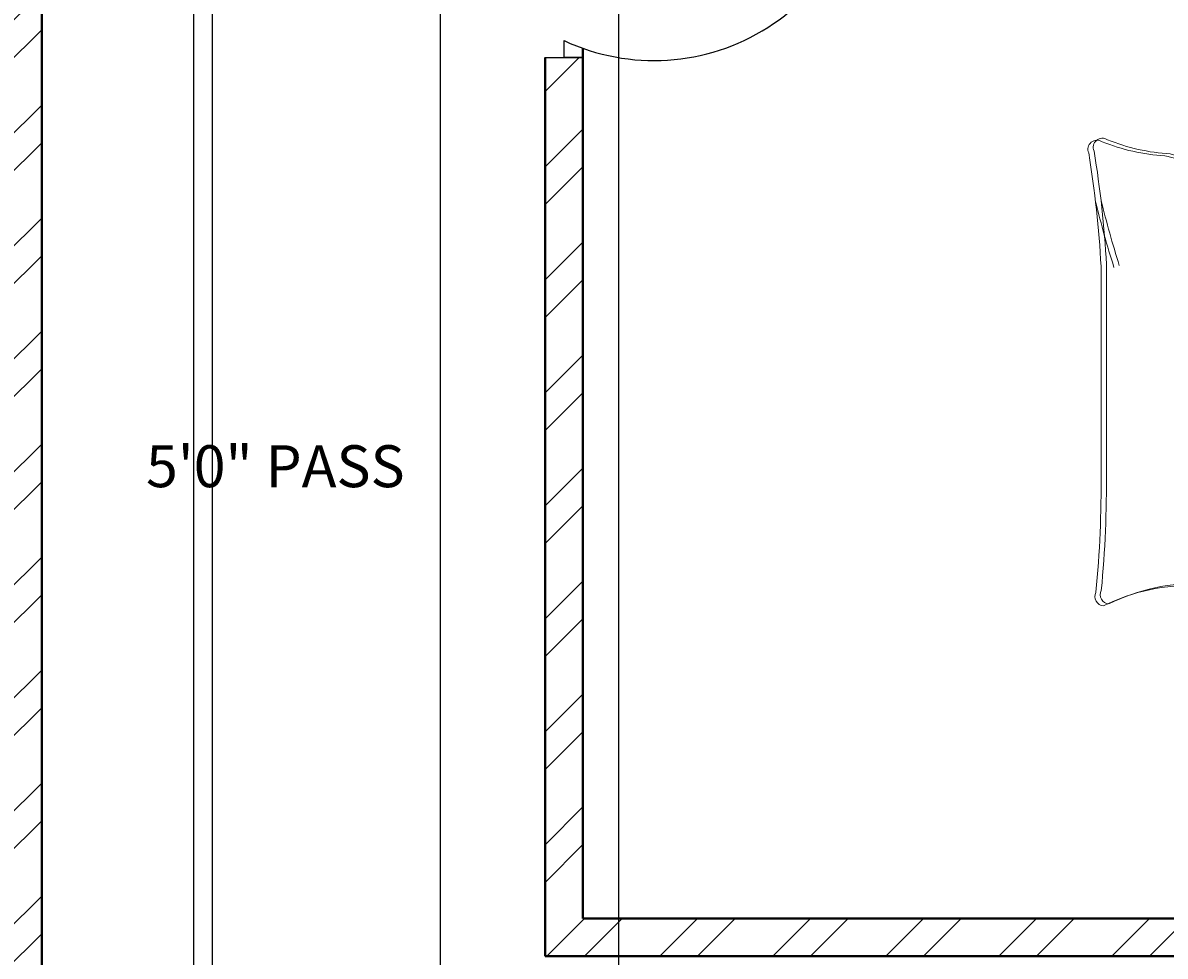
# Model space of a CAD drawing. Units: inches. Extents: x 2063 to 2617, y 1299 to 2210.
# Tile 15 of 22: x 2338 to 2475, y 1727 to 1839. Entities that reach past the tile are written whole.
import ezdxf

# ---------------------------------------------------------------- set-up
doc = ezdxf.new("R2010")
doc.units = ezdxf.units.IN
for name, color, linetype, lineweight in [('A-ANNO-DIMS', 2, 'Continuous', 18), ('A-AREA-IDEN', 7, 'Continuous', 18), ('A-DOOR', 11, 'Continuous', 25), ('A-FURN', 8, 'Continuous', 18), ('A-WALL', 7, 'Continuous', 40)]:
    doc.layers.add(name, color=color, linetype=linetype, lineweight=lineweight)
doc.layers.add('A-WALL-PATT', color=215, linetype='Continuous', lineweight=13, true_color=0xa953a0)
doc.styles.get("Standard").update_dxf_attribs({"font": 'arial.ttf'})
doc.dimstyles.get("Standard").update_dxf_attribs({"dimtxt": 0.18, "dimasz": 0.18, "dimexe": 0.18, "dimexo": 0.0625, "dimgap": 0.09, "dimtad": 0, "dimtih": 1, "dimtoh": 1, "dimdec": 4, "dimzin": 0, "dimdsep": 46, "dimtxsty": 'Standard', "dimcen": 0.09, "dimadec": 0, "dimazin": 0, "dimtfac": 1, "dimtdec": 4, "dimtofl": 0, "dimtmove": 0, "dimatfit": 3, "dimfxl": 1, "dimtolj": 1, "dimtzin": 0, "dimarcsym": 0})

# ---------------------------------------------------------------- blocks, each defined once
blk = doc.blocks.new('BED-DOUBLE')
for p, q in [((3.48, 63.33), (3.48, 81.44)), ((3.48, 63.33), (3.48, 81.44)), ((3.48, 81.44), (51.49, 81.44)), ((3.7, 62.69), (3.7, 80.8)), ((3.7, 62.69), (3.7, 80.8)), ((51.27, 81.44), (51.27, 54.83)), ((51.27, 81.44), (51.27, 54.83)), ((51.49, 81.44), (51.49, 80.8)), ((51.49, 80.8), (51.49, 54.19)), ((51.49, 80.8), (51.49, 54.19)), ((3.48, 79.91), (51.27, 79.91)), ((3.48, 79.91), (51.27, 79.91)), ((3.7, 79.27), (51.49, 79.27)), ((3.7, 79.27), (51.49, 79.27)), ((16.88, 78.42), (19.77, 79.14)), ((16.88, 78.42), (19.77, 79.14)), ((19.77, 79.14), (20.09, 79.14)), ((19.77, 79.14), (20.09, 79.14)), ((20.09, 79.14), (24.54, 79)), ((20.09, 79.14), (24.54, 79)), ((24.54, 79), (25.98, 79.57)), ((24.54, 79), (25.98, 79.57)), ((25.98, 79.57), (26.56, 74.22)), ((25.98, 79.57), (26.56, 74.22)), ((50.11, 78.89), (44.71, 78.98)), ((44.71, 78.98), (45.71, 78.9)), ((50.11, 78.89), (44.71, 78.98)), ((44.71, 78.98), (45.71, 78.9)), ((3.89, 78.13), (4.47, 74.95)), ((3.9, 78.11), (8.18, 78.43)), ((3.9, 78.11), (8.18, 78.43)), ((3.9, 78.13), (4.47, 74.95)), ((4.13, 77.47), (8.41, 77.8)), ((4.13, 77.47), (8.41, 77.8)), ((8.18, 78.43), (8.29, 78.42)), ((8.18, 78.43), (8.29, 78.42)), ((8.29, 78.42), (12.11, 78.13)), ((8.29, 78.42), (12.11, 78.13)), ((8.41, 77.8), (8.51, 77.78)), ((8.41, 77.8), (8.51, 77.78)), ((8.51, 77.78), (12.34, 77.49)), ((8.51, 77.78), (12.34, 77.49)), ((12.11, 78.13), (17.6, 77.12)), ((12.11, 78.13), (17.6, 77.12)), ((14.86, 77.69), (16.88, 78.42)), ((14.86, 77.69), (16.88, 78.42)), ((15.08, 77.05), (17.11, 77.78)), ((15.08, 77.05), (17.11, 77.78)), ((17.11, 77.78), (20, 78.5)), ((17.11, 77.78), (20, 78.5)), ((20, 78.5), (20.32, 78.5)), ((20, 78.5), (20.32, 78.5)), ((20.32, 78.5), (24.77, 78.36)), ((20.32, 78.5), (24.77, 78.36)), ((24.77, 78.36), (26.21, 78.93)), ((24.77, 78.36), (26.21, 78.93)), ((26.21, 78.93), (26.79, 73.58)), ((26.21, 78.93), (26.79, 73.58)), ((27.98, 78.95), (27.73, 73.58)), ((27.98, 78.95), (27.73, 73.58)), ((28.21, 78.31), (27.96, 72.94)), ((28.21, 78.31), (27.96, 72.94)), ((29.46, 78.46), (27.98, 78.95)), ((29.46, 78.46), (27.98, 78.95)), ((29.68, 77.83), (28.21, 78.31)), ((29.68, 77.83), (28.21, 78.31)), ((33.88, 78.89), (29.46, 78.46)), ((33.88, 78.89), (29.46, 78.46)), ((34.11, 78.25), (29.68, 77.83)), ((34.11, 78.25), (29.68, 77.83)), ((34.21, 78.91), (33.88, 78.89)), ((34.2, 78.91), (33.88, 78.89)), ((34.43, 78.27), (34.11, 78.25)), ((34.43, 78.27), (34.11, 78.25)), ((37.14, 78.37), (34.2, 78.91)), ((37.14, 78.37), (34.21, 78.91)), ((37.36, 77.73), (34.43, 78.27)), ((37.36, 77.73), (34.43, 78.27)), ((41.91, 78.37), (36.5, 77.02)), ((41.91, 78.37), (36.5, 77.02)), ((42.14, 77.73), (36.72, 76.38)), ((42.14, 77.73), (36.72, 76.38)), ((39.2, 77.77), (37.14, 78.37)), ((39.2, 77.77), (37.14, 78.37)), ((39.43, 77.13), (37.36, 77.73)), ((39.43, 77.13), (37.36, 77.73)), ((45.71, 78.9), (41.91, 78.37)), ((45.71, 78.9), (41.91, 78.37)), ((45.94, 78.26), (42.14, 77.73)), ((45.94, 78.26), (42.14, 77.73)), ((50.34, 78.25), (44.94, 78.34)), ((44.94, 78.34), (45.94, 78.26)), ((50.34, 78.25), (44.94, 78.34)), ((44.94, 78.34), (45.94, 78.26)), ((50.11, 78.89), (49.73, 75.68)), ((50.11, 78.89), (49.73, 75.68)), ((50.34, 78.25), (49.96, 75.04)), ((50.34, 78.25), (49.96, 75.04)), ((4.12, 77.49), (4.7, 74.31)), ((4.12, 77.49), (4.7, 74.31)), ((12.34, 77.49), (17.83, 76.48)), ((12.34, 77.49), (17.83, 76.48)), ((4.47, 74.95), (4.04, 72.34)), ((4.47, 74.95), (4.04, 72.34)), ((5.05, 72.49), (6.06, 75.24)), ((5.05, 72.49), (6.06, 75.24)), ((49.31, 73.19), (48.13, 75.87)), ((49.31, 73.19), (48.13, 75.87)), ((49.54, 72.55), (48.36, 75.23)), ((49.54, 72.55), (48.36, 75.23)), ((49.73, 75.68), (50.33, 73.11)), ((49.73, 75.68), (50.33, 73.11)), ((49.96, 75.04), (50.56, 72.47)), ((49.96, 75.04), (50.56, 72.47)), ((4.7, 74.31), (4.27, 71.7)), ((4.7, 74.31), (4.27, 71.7)), ((5.28, 71.85), (6.29, 74.6)), ((5.28, 71.85), (6.29, 74.6)), ((26.56, 74.22), (27.14, 71.04)), ((26.56, 74.22), (27.14, 71.04)), ((26.79, 73.58), (27.37, 70.4)), ((26.79, 73.58), (27.37, 70.4)), ((27.73, 73.58), (27.36, 70.37)), ((27.73, 73.58), (27.36, 70.37)), ((4.04, 72.34), (4.62, 71.33)), ((4.04, 72.34), (4.62, 71.33)), ((4.47, 68.87), (5.05, 72.49)), ((4.47, 68.87), (5.05, 72.49)), ((27.96, 72.94), (27.58, 69.73)), ((27.96, 72.94), (27.58, 69.73)), ((50.11, 69.61), (49.31, 73.19)), ((50.11, 69.61), (49.31, 73.19)), ((50.34, 68.98), (49.54, 72.55)), ((50.34, 68.98), (49.54, 72.55)), ((50.33, 73.11), (49.81, 72.06)), ((50.33, 73.11), (49.82, 72.06)), ((50.56, 72.47), (50.04, 71.42)), ((50.56, 72.47), (50.04, 71.42)), ((4.27, 71.7), (4.85, 70.69)), ((4.27, 71.7), (4.85, 70.69)), ((4.7, 68.23), (5.28, 71.85)), ((4.7, 68.23), (5.28, 71.85)), ((27.14, 71.04), (27.14, 69.74)), ((27.14, 71.04), (27.14, 69.74)), ((27.14, 69.74), (26.56, 67.86)), ((27.14, 69.74), (26.56, 67.86)), ((27.36, 70.37), (27.44, 69.07)), ((27.36, 70.37), (27.44, 69.07)), ((27.37, 70.4), (27.37, 69.1)), ((27.37, 70.4), (27.37, 69.1)), ((27.58, 69.73), (27.66, 68.43)), ((27.58, 69.73), (27.66, 68.43)), ((49.92, 68.01), (50.11, 69.61)), ((49.92, 68.01), (50.11, 69.61)), ((4.76, 67.28), (4.47, 68.87)), ((4.76, 67.28), (4.47, 68.87)), ((4.99, 66.64), (4.7, 68.23)), ((4.99, 66.64), (4.7, 68.23)), ((27.37, 69.1), (26.79, 67.22)), ((27.37, 69.1), (26.79, 67.22)), ((27.44, 69.07), (28.13, 67.23)), ((27.44, 69.07), (28.13, 67.23)), ((27.66, 68.43), (28.36, 66.59)), ((27.66, 68.43), (28.36, 66.59)), ((50.15, 67.37), (50.34, 68.98)), ((50.15, 67.37), (50.34, 68.98)), ((4.18, 64.1), (4.76, 67.28)), ((4.18, 64.1), (4.76, 67.28)), ((26.56, 67.86), (26.56, 65.18)), ((26.56, 67.86), (26.56, 65.18)), ((26.79, 67.22), (26.79, 64.54)), ((26.79, 67.22), (26.79, 64.54)), ((28.13, 67.23), (28.3, 64.55)), ((28.13, 67.23), (28.3, 64.55)), ((50.7, 64.87), (49.92, 68.01)), ((50.7, 64.87), (49.92, 68.01)), ((50.93, 64.23), (50.15, 67.37)), ((50.93, 64.23), (50.15, 67.37)), ((4.41, 63.46), (4.99, 66.64)), ((4.41, 63.46), (4.99, 66.64)), ((6.38, 65.82), (10.41, 65.15)), ((6.38, 65.82), (10.41, 65.15)), ((24.1, 65.18), (20.96, 66.27)), ((24.1, 65.18), (20.96, 66.27)), ((24.33, 64.54), (21.19, 65.63)), ((24.33, 64.54), (21.19, 65.63)), ((28.36, 66.59), (28.53, 63.91)), ((28.36, 66.59), (28.53, 63.91)), ((30.75, 64.7), (33.82, 65.99)), ((30.75, 64.7), (33.82, 65.99)), ((30.98, 64.06), (34.05, 65.35)), ((30.98, 64.06), (34.05, 65.35)), ((32.56, 65.82), (36.6, 65.15)), ((32.56, 65.82), (36.6, 65.15)), ((9.28, 64.83), (4.18, 64.1)), ((9.28, 64.83), (4.18, 64.1)), ((9.51, 64.19), (4.41, 63.46)), ((9.51, 64.19), (4.41, 63.46)), ((6.61, 65.18), (10.64, 64.51)), ((6.61, 65.18), (10.64, 64.51)), ((10.41, 65.15), (9.28, 64.83)), ((10.41, 65.15), (9.28, 64.83)), ((10.64, 64.51), (9.51, 64.19)), ((10.64, 64.51), (9.51, 64.19)), ((10.41, 65.15), (17.42, 64.72)), ((10.41, 65.15), (17.42, 64.72)), ((10.64, 64.51), (17.65, 64.08)), ((10.64, 64.51), (17.65, 64.08)), ((17.42, 64.72), (19.38, 65.27)), ((17.42, 64.72), (19.38, 65.27)), ((17.65, 64.08), (19.61, 64.64)), ((17.65, 64.08), (19.61, 64.64)), ((19.38, 65.27), (24.52, 64.87)), ((19.38, 65.27), (24.52, 64.87)), ((19.61, 64.64), (24.74, 64.23)), ((19.61, 64.64), (24.74, 64.23)), ((26.56, 65.18), (24.1, 65.18)), ((26.56, 65.18), (24.1, 65.18)), ((26.79, 64.54), (24.33, 64.54)), ((26.79, 64.54), (24.33, 64.54)), ((28.3, 64.55), (30.75, 64.7)), ((28.3, 64.55), (30.75, 64.7)), ((28.53, 63.91), (30.98, 64.06)), ((28.53, 63.91), (30.98, 64.06)), ((30.26, 64.06), (34.45, 57.57)), ((30.26, 64.06), (34.45, 57.57)), ((40.64, 61.13), (32.31, 64.06)), ((40.64, 61.13), (32.31, 64.06)), ((32.79, 65.18), (36.83, 64.51)), ((32.79, 65.18), (36.82, 64.51)), ((36.6, 65.15), (43.61, 64.72)), ((36.6, 65.15), (43.61, 64.72)), ((36.82, 64.51), (43.83, 64.08)), ((36.83, 64.51), (43.84, 64.08)), ((43.61, 64.72), (45.57, 65.27)), ((43.61, 64.72), (45.57, 65.27)), ((43.83, 64.08), (45.8, 64.64)), ((43.84, 64.08), (45.8, 64.64)), ((45.57, 65.27), (50.7, 64.87)), ((45.57, 65.27), (50.7, 64.87)), ((45.8, 64.64), (50.93, 64.23)), ((45.8, 64.64), (50.93, 64.23)), ((30.49, 63.42), (34.68, 56.93)), ((30.49, 63.42), (34.68, 56.93)), ((40.87, 60.49), (32.53, 63.42)), ((40.87, 60.49), (32.54, 63.42)), ((46.22, 59.11), (40.64, 61.13)), ((46.22, 59.11), (40.64, 61.13)), ((46.45, 58.48), (40.87, 60.49)), ((46.45, 58.48), (40.87, 60.49)), ((49.16, 56.95), (46.22, 59.11)), ((49.16, 56.95), (46.22, 59.11)), ((34.45, 57.57), (36.15, 53.08)), ((34.45, 57.57), (36.15, 53.08)), ((49.39, 56.31), (46.45, 58.48)), ((49.39, 56.31), (46.45, 58.48)), ((34.68, 56.93), (36.38, 52.44)), ((34.68, 56.93), (36.38, 52.44)), ((52.87, 53.7), (49.16, 56.95)), ((52.87, 53.7), (49.16, 56.95)), ((53.1, 53.06), (49.39, 56.31)), ((53.1, 53.06), (49.39, 56.31)), ((44.36, 53.08), (48.23, 53.39)), ((44.36, 53.08), (48.23, 53.39)), ((48.23, 53.39), (51.33, 53.08)), ((48.23, 53.39), (51.33, 53.08)), ((51.33, 53.08), (52.87, 53.7)), ((51.33, 53.08), (52.87, 53.7)), ((52.95, 51.95), (52.87, 53.7, 3.87)), ((52.95, 51.95), (52.87, 53.7, 3.87)), ((36.15, 53.08), (36.46, 51.07)), ((36.15, 53.08), (36.46, 51.07)), ((36.38, 52.44), (36.69, 50.43)), ((36.38, 52.44), (36.69, 50.43)), ((38.94, 51.69), (40.95, 52.61)), ((38.94, 51.69), (40.95, 52.61)), ((39.17, 51.05), (41.18, 51.97)), ((39.17, 51.05), (41.18, 51.97)), ((40.95, 52.61), (44.36, 53.08)), ((40.95, 52.61), (44.36, 53.08)), ((41.18, 51.97), (44.59, 52.44)), ((41.18, 51.97), (44.59, 52.44)), ((44.59, 52.44), (48.46, 52.75)), ((44.59, 52.44), (48.46, 52.75)), ((48.46, 52.75), (51.56, 52.44)), ((48.46, 52.75), (51.56, 52.44)), ((51.56, 52.44), (53.1, 53.06)), ((51.56, 52.44), (53.1, 53.06)), ((53.18, 51.31), (53.1, 53.06, 3.87)), ((53.18, 51.31), (53.1, 53.06, 3.87)), ((36.46, 51.07), (38.94, 51.69)), ((36.46, 51.07), (38.94, 51.69)), ((36.69, 50.43), (39.17, 51.05)), ((36.69, 50.43), (39.17, 51.05)), ((15.06, 2.2), (39.68, 2.2)), ((15.06, 2.2), (39.68, 2.2)), ((15.29, 1.56), (39.91, 1.56)), ((15.29, 1.56), (39.91, 1.56))]:
    blk.add_line(p, q)
for centre, radius, start, end in [((21.36, -100.61), 164.97, 86.0865, 96.7821), ((21.36, -100.61), 164.97, 86.0865, 96.7821), ((85.16, 61.35), 83.31, 178.7218, 185.604), ((85.16, 61.35), 83.31, 178.7218, 185.604), ((21.59, -101.25), 164.97, 86.0865, 96.7821), ((21.59, -101.25), 164.97, 86.0865, 96.7821), ((85.39, 60.71), 83.31, 178.7218, 185.604), ((85.39, 60.71), 83.31, 178.7218, 185.604), ((17.76, -74.87), 129.02, 81.7845, 96.9006), ((17.76, -74.87), 129.02, 81.7845, 96.9006), ((17.98, -75.51), 129.02, 81.7845, 96.9006), ((17.98, -75.51), 129.02, 81.7845, 96.9006), ((-167.31, 50.27), 170.11, 358.4762, 1.0082), ((-167.31, 50.27), 170.11, 358.4762, 1.0082), ((-167.08, 49.63), 170.11, 358.4762, 1.0082), ((-167.08, 49.63), 170.11, 358.4762, 1.0082), ((31.15, 79.96), 29.65, 280.6617, 289.8806), ((31.15, 79.96), 29.65, 280.6617, 289.8806), ((43.74, 46.38), 6.22, 78.6608, 113.7384), ((43.74, 46.38), 6.22, 78.6608, 113.7384), ((43.97, 45.74), 6.22, 78.6608, 113.7384), ((43.97, 45.74), 6.22, 78.6608, 113.7384), ((51.33, 88.1), 36.18, 259.8763, 272.5657), ((51.33, 88.1), 36.18, 259.8763, 272.5657), ((51.56, 87.46), 36.18, 259.8763, 272.5657), ((51.56, 87.46), 36.18, 259.8763, 272.5657), ((182.27, 45.13), 129.5, 176.9791, 183.8365), ((182.27, 45.13), 129.5, 176.9791, 183.8365), ((36.64, 51), 0.185, 160.2464, 271.1377), ((36.64, 51), 0.185, 160.2464, 271.1377), ((36.87, 50.36), 0.185, 160.2464, 271.1377), ((36.86, 50.36), 0.185, 160.2464, 271.1377), ((31.38, 79.32), 29.65, 280.6617, 289.8806), ((31.38, 79.32), 29.65, 280.6617, 289.8806), ((182.49, 44.49), 129.5, 176.9791, 183.8365), ((182.49, 44.49), 129.5, 176.9791, 183.8365), ((484.82, 30.83), 482.31, 178.2277, 181.7185), ((484.82, 30.83), 482.31, 178.2277, 181.7185), ((485.05, 30.19), 482.31, 178.2277, 181.7185), ((485.05, 30.19), 482.31, 178.2277, 181.7185), ((-4508.74, 13.62), 4561.86, 0.00217, 0.28689), ((-4508.74, 13.62), 4561.86, 0.00217, 0.28689), ((-4508.51, 12.98), 4561.86, 0.00217, 0.28689), ((-4508.51, 12.98), 4561.86, 0.00217, 0.28689), ((-26.9, 16.93), 29.63, 346.0648, 358.9113), ((-26.9, 16.93), 29.63, 346.0648, 358.9113), ((-26.67, 16.29), 29.63, 346.0648, 358.9113), ((-26.67, 16.29), 29.63, 346.0648, 358.9113), ((76.16, 12.78), 23.07, 177.4714, 206.4681), ((76.16, 12.78), 23.07, 177.4714, 206.4681), ((76.39, 12.14), 23.07, 177.4714, 206.4681), ((76.39, 12.14), 23.07, 177.4714, 206.4681), ((-21.66, 11.17), 23.56, 337.9751, 356.652), ((-21.66, 11.17), 23.56, 337.9751, 356.652), ((-21.43, 10.53), 23.56, 337.9751, 356.652), ((-21.43, 10.53), 23.56, 337.9751, 356.652), ((-17.22, 105.16), 106.46, 283.3832, 287.7053), ((-17.22, 105.16), 106.46, 283.3832, 287.7053), ((-16.99, 104.52), 106.46, 283.3832, 287.7053), ((-16.99, 104.52), 106.46, 283.3832, 287.7053), ((1.09, 1.73), 1.09, 146.1736, 293.4781), ((1.09, 1.73), 1.09, 146.1736, 293.4781), ((1.32, 1.09), 1.09, 146.1736, 293.4781), ((1.32, 1.09), 1.09, 146.1736, 293.4781), ((21.43, -119.39), 121.76, 92.9958, 99.4091), ((21.43, -119.39), 121.76, 92.9958, 99.4091), ((21.66, -120.03), 121.76, 92.9958, 99.4091), ((21.66, -120.03), 121.76, 92.9958, 99.4091), ((41.15, -130.83), 133.04, 84.4998, 90.6351), ((41.15, -130.83), 133.04, 84.4998, 90.6351), ((41.38, -131.47), 133.04, 84.4998, 90.6351), ((41.38, -131.47), 133.04, 84.4998, 90.6351), ((54.41, 2.57), 1.1, 242.6588, 356.02), ((54.41, 2.57), 1.1, 242.6588, 356.02), ((54.64, 1.93), 1.1, 242.6588, 356.02), ((54.64, 1.93), 1.1, 242.6588, 356.02)]:
    blk.add_arc(centre, radius, start, end)
blk = doc.blocks.new('*D51')
at = {"layer": 'A-ANNO-DIMS', "color": 0, "lineweight": -2, "transparency": 16777216}
for p, q in [((2340.64, 2124.25), (2340.64, 1317.7)), ((2358.75, 2124.25), (2358.75, 1317.7)), ((2340.82, 1317.88), (2349.24, 1317.88)), ((2358.57, 1317.88), (2350.15, 1317.88))]:
    blk.add_line(p, q, dxfattribs=at)
at = {"layer": 'A-ANNO-DIMS', "color": 0, "transparency": 16777216}
for points in [[(2340.82, 1317.91), (2340.82, 1317.85), (2340.64, 1317.88)], [(2358.57, 1317.91), (2358.57, 1317.85), (2358.75, 1317.88)]]:
    blk.add_solid(points, dxfattribs=at)
at = {"layer": 'Defpoints', "color": 0, "transparency": 16777216}
for p in [(2340.64, 2124.31), (2358.75, 2124.31), (2358.75, 1317.88)]:
    blk.add_point(p, dxfattribs=at)
at = {"layer": 'A-ANNO-DIMS', "color": 0, "transparency": 16777216, "insert": (2349.7, 1317.88), "char_height": 0.18, "attachment_point": 5}
blk.add_mtext('\\A1;18.106', dxfattribs=at)
blk = doc.blocks.new('*D54')
at = {"layer": 'A-ANNO-DIMS', "color": 0, "lineweight": -2, "transparency": 16777216}
for p, q in [((2340.64, 2124.25), (2340.64, 1317.7)), ((2360.96, 2104.46), (2360.96, 1317.7)), ((2340.82, 1317.88), (2350.34, 1317.88)), ((2360.78, 1317.88), (2351.27, 1317.88))]:
    blk.add_line(p, q, dxfattribs=at)
at = {"layer": 'A-ANNO-DIMS', "color": 0, "transparency": 16777216}
for points in [[(2340.82, 1317.91), (2340.82, 1317.85), (2340.64, 1317.88)], [(2360.78, 1317.91), (2360.78, 1317.85), (2360.96, 1317.88)]]:
    blk.add_solid(points, dxfattribs=at)
at = {"layer": 'Defpoints', "color": 0, "transparency": 16777216}
for p in [(2340.64, 2124.31), (2360.96, 2104.52), (2360.96, 1317.88)]:
    blk.add_point(p, dxfattribs=at)
at = {"layer": 'A-ANNO-DIMS', "color": 0, "transparency": 16777216, "insert": (2350.8, 1317.88), "char_height": 0.18, "attachment_point": 5}
blk.add_mtext('\\A1;20.317', dxfattribs=at)
blk = doc.blocks.new('*D55')
at = {"layer": 'A-ANNO-DIMS', "color": 0, "lineweight": -2, "transparency": 16777216}
for p, q in [((2388.15, 1975.75), (2388.15, 1317.7)), ((2409.37, 1975.75), (2409.37, 1317.7)), ((2388.33, 1317.88), (2398.3, 1317.88)), ((2409.19, 1317.88), (2399.23, 1317.88))]:
    blk.add_line(p, q, dxfattribs=at)
at = {"layer": 'A-ANNO-DIMS', "color": 0, "transparency": 16777216}
for points in [[(2388.33, 1317.91), (2388.33, 1317.85), (2388.15, 1317.88)], [(2409.19, 1317.91), (2409.19, 1317.85), (2409.37, 1317.88)]]:
    blk.add_solid(points, dxfattribs=at)
at = {"layer": 'Defpoints', "color": 0, "transparency": 16777216}
for p in [(2388.15, 1975.81), (2409.37, 1975.81), (2409.37, 1317.88)]:
    blk.add_point(p, dxfattribs=at)
at = {"layer": 'A-ANNO-DIMS', "color": 0, "transparency": 16777216, "insert": (2398.76, 1317.88), "char_height": 0.18, "attachment_point": 5}
blk.add_mtext('\\A1;21.225', dxfattribs=at)
blk = doc.blocks.new('*D59')
at = {"layer": 'A-ANNO-DIMS', "color": 0, "lineweight": -2, "transparency": 16777216}
for p, q in [((2290.14, 1554.56), (2290.14, 2170.74)), ((2290.32, 2170.56), (2315.07, 2170.56)), ((2340.46, 2170.56), (2315.72, 2170.56)), ((2340.64, 1554.56), (2340.64, 2170.74))]:
    blk.add_line(p, q, dxfattribs=at)
at = {"layer": 'A-ANNO-DIMS', "color": 0, "transparency": 16777216}
for points in [[(2290.32, 2170.59), (2290.32, 2170.53), (2290.14, 2170.56)], [(2340.46, 2170.59), (2340.46, 2170.53), (2340.64, 2170.56)]]:
    blk.add_solid(points, dxfattribs=at)
at = {"layer": 'Defpoints', "color": 0, "transparency": 16777216}
for p in [(2340.64, 2170.56), (2290.14, 1554.5), (2340.64, 1554.5)]:
    blk.add_point(p, dxfattribs=at)
at = {"layer": 'A-ANNO-DIMS', "color": 0, "transparency": 16777216, "insert": (2315.39, 2170.56), "char_height": 0.18, "attachment_point": 5}
blk.add_mtext('\\A1;50.5', dxfattribs=at)

msp = doc.modelspace()

# ---------------------------------------------------------------- hatches: boundary and pattern name
at = {"layer": 'A-WALL-PATT'}
h = msp.add_hatch(dxfattribs=at)
h.set_pattern_fill('ANSI32', color=256)
h.paths.add_polyline_path([(2553.6442, 2128.8122), (2511.1703, 2128.8122), (2511.1703, 2124.3122), (2549.1442, 2124.3122), (2549.1442, 2095.662), (2553.6442, 2095.662)])
h.paths.add_polyline_path([(2553.6442, 2035.662), (2549.1442, 2035.662), (2549.1442, 1980.3122), (2503.7214, 1980.3122), (2503.7214, 1975.8122), (2549.1442, 1975.8122), (2549.1442, 1962.9693), (2553.6442, 1962.9693)])
h.paths.add_polyline_path([(2553.6442, 1938.9693), (2549.1442, 1938.9693), (2549.1442, 1927.8122), (2477.1442, 1927.8122), (2477.1442, 1975.8122), (2481.2918, 1975.8122), (2481.2918, 1980.3122), (2453.2648, 1980.3122), (2453.2648, 1975.8122), (2472.6442, 1975.8122), (2472.6442, 1868.3122), (2400.6442, 1868.3122), (2400.6442, 1861.3782), (2405.1442, 1861.3782), (2405.1442, 1863.8122), (2480.9699, 1863.8122), (2480.9699, 1866.0622), (2480.9699, 1868.3122), (2477.1442, 1868.3122), (2477.1442, 1923.3122), (2549.1442, 1923.3122), (2549.1442, 1908.8504), (2553.6442, 1908.8504)])
h.paths.add_polyline_path([(2553.6442, 1884.8504), (2549.1442, 1884.8504), (2549.1442, 1868.3122), (2501.0636, 1868.3122), (2501.0636, 1863.8122), (2549.1442, 1863.8122), (2549.1442, 1826.0298), (2553.6442, 1826.0298)])
h.paths.add_polyline_path([(2388.1504, 1980.3122), (2340.6442, 1980.3122), (2340.6442, 2124.3122), (2358.7501, 2124.3122), (2358.7501, 2128.8122), (2316.3482, 2128.8122), (2316.3482, 2124.3122), (2336.1442, 2124.3122), (2336.1442, 1980.3122), (2289.1737, 1980.3122), (2289.1737, 1975.8122), (2336.1442, 1975.8122), (2336.1442, 1619.3122), (2333.1433, 1619.3122), (2333.1433, 1614.8122), (2344.1671, 1614.8122), (2344.1671, 1617.0622), (2344.1671, 1619.3122), (2340.6442, 1619.3122), (2340.6442, 1975.8122), (2388.1504, 1975.8122), (2388.1504, 1978.0622)])
h.paths.add_polyline_path([(2290.1442, 1614.8122), (2301.4594, 1614.8122), (2301.4594, 1617.0622), (2301.4594, 1619.3122), (2285.6442, 1619.3122), (2285.6442, 1566.8122), (2280.8619, 1566.8122), (2280.8619, 1564.5622), (2280.8619, 1562.3122), (2285.6442, 1562.3122), (2285.6442, 1442.3122), (2281.7879, 1442.3122), (2281.7879, 1437.8122), (2285.6442, 1437.8122), (2285.6442, 1401.8122), (2290.1442, 1401.8122)])
h.paths.add_polyline_path([(2549.1442, 1731.8122), (2405.1442, 1731.8122), (2405.1442, 1834.4638), (2402.8942, 1834.4638), (2400.6442, 1834.4638), (2400.6442, 1727.3122), (2549.1442, 1727.3122)])
h.paths.add_polyline_path([(2553.6442, 1766.0298), (2551.3942, 1766.0298), (2549.1442, 1766.0298), (2549.1442, 1686.7767), (2553.6442, 1686.7767)])
h.paths.add_polyline_path([(2553.6442, 1638.7767), (2551.3942, 1638.7767), (2549.1442, 1638.7767), (2549.1442, 1619.3122), (2448.6442, 1619.3122), (2448.6442, 1610.5671), (2450.8942, 1610.5671), (2453.1442, 1610.5671), (2453.1442, 1614.8122), (2549.1442, 1614.8122), (2549.1442, 1601.6421), (2553.6442, 1601.6421)])
h.paths.add_polyline_path([(2553.6442, 1577.6421), (2551.3942, 1577.6421), (2549.1442, 1577.6421), (2549.1442, 1566.8122), (2453.1442, 1566.8122), (2453.1442, 1591.5045), (2451.0335, 1591.5045), (2448.6442, 1591.5045), (2448.6442, 1566.8122), (2434.0475, 1566.8122), (2434.0475, 1562.3122), (2549.1442, 1562.3122), (2549.1442, 1533.48), (2553.6442, 1533.48)])
h.paths.add_polyline_path([(2553.6442, 1473.48), (2549.1442, 1473.48), (2549.1442, 1442.3122), (2502.6258, 1442.3122), (2502.6258, 1437.8122), (2549.1442, 1437.8122), (2549.1442, 1401.8122), (2553.6442, 1401.8122)])
h.paths.add_polyline_path([(2395.6442, 1562.3122), (2400.0901, 1562.3122), (2400.0901, 1564.5622), (2400.0901, 1566.8122), (2395.6442, 1566.8122), (2395.6442, 1619.3122), (2379.1127, 1619.3122), (2379.1127, 1614.8122), (2391.1442, 1614.8122), (2391.1442, 1401.8122), (2395.6442, 1401.8122), (2395.6442, 1437.8122), (2399.2425, 1437.8122), (2399.2425, 1440.0622), (2399.2425, 1442.3122), (2395.6442, 1442.3122)])
h.paths.add_polyline_path([(2442.6258, 1442.3122), (2419.6262, 1442.3122), (2419.6262, 1437.8122), (2442.6258, 1437.8122), (2442.6258, 1440.0622)])
h.paths.add_polyline_path([(2127.6442, 1480.2532), (2125.3942, 1480.2532), (2123.1442, 1480.2532), (2123.1442, 1401.8122), (2127.6442, 1401.8122), (2127.6442, 1437.8122), (2145.1538, 1437.8122), (2145.1538, 1440.0622), (2145.1538, 1442.3122), (2127.6442, 1442.3122)])
h.paths.add_polyline_path([(2259.809, 1442.3122), (2205.1538, 1442.3122), (2205.1538, 1437.8122), (2259.809, 1437.8122), (2259.809, 1440.0622)])
h.paths.add_polyline_path([(2127.6442, 1659.7652), (2123.1442, 1659.7652), (2123.1442, 1605.5161), (2125.3942, 1605.5161), (2127.6442, 1605.5161), (2127.6442, 1614.8122), (2223.6442, 1614.8122), (2223.6442, 1611.2723), (2228.1442, 1611.2723), (2228.1442, 1619.3122), (2127.6442, 1619.3122)])
h.paths.add_polyline_path([(2244.8673, 1566.8122), (2228.1442, 1566.8122), (2228.1442, 1590.8122), (2225.8942, 1590.8122), (2223.6442, 1590.8122), (2223.6442, 1566.8122), (2127.6442, 1566.8122), (2127.6442, 1581.5161), (2123.1442, 1581.5161), (2123.1442, 1540.2532), (2127.6442, 1540.2532), (2127.6442, 1562.3122), (2244.8673, 1562.3122), (2244.8673, 1564.5622)])
h.paths.add_polyline_path([(2172.5174, 1868.3122), (2127.6442, 1868.3122), (2127.6442, 1886.5833), (2123.1442, 1886.5833), (2123.1442, 1832.6633), (2127.6442, 1832.6633), (2127.6442, 1863.8122), (2172.5174, 1863.8122), (2172.5174, 1866.0622)])
h.paths.add_polyline_path([(2276.1442, 1868.3122), (2204.1442, 1868.3122), (2204.1442, 1923.3122), (2204.1442, 1975.8122), (2224.8362, 1975.8122), (2224.8362, 1978.1097), (2224.8362, 1980.3122), (2195.0729, 1980.3122), (2195.0729, 1978.0622), (2195.0729, 1975.8122), (2199.6442, 1975.8122), (2199.6442, 1927.8122), (2127.6442, 1927.8122), (2127.6442, 1942.3492), (2123.1442, 1942.3492), (2123.1442, 1910.5833), (2127.6442, 1910.5833), (2127.6442, 1923.3122), (2199.6442, 1923.3122), (2199.6442, 1868.3122), (2194.8228, 1868.3122), (2194.8228, 1864.7337), (2194.8228, 1863.8122), (2271.6442, 1863.8122), (2271.6442, 1860.0507), (2276.1442, 1860.0507)])
h.paths.add_polyline_path([(2276.1442, 1829.994), (2273.8942, 1829.994), (2271.6442, 1829.994), (2271.6442, 1731.8122), (2127.6442, 1731.8122), (2127.6442, 1772.6633), (2123.1442, 1772.6633), (2123.1442, 1707.7652), (2127.6442, 1707.7652), (2127.6442, 1727.3122), (2276.1442, 1727.3122)])
h.paths.add_polyline_path([(2127.6442, 2022.1152), (2123.1442, 2022.1152), (2123.1442, 1966.3492), (2127.6442, 1966.3492), (2127.6442, 1975.8122), (2174.2082, 1975.8122), (2174.2082, 1978.0622), (2174.2082, 1980.3122), (2127.6442, 1980.3122)])
h.paths.add_polyline_path([(2361.9755, 1678.588), (2398.4558, 1678.588), (2398.4558, 1697.2453), (2361.9755, 1697.2453)], flags=9)
h.paths.add_polyline_path([(2351.5397, 1780.4072), (2386.1987, 1780.4072), (2386.1987, 1790.7107), (2351.5397, 1790.7107)], flags=25)
h.paths.add_polyline_path([(2350.6753, 1940.9321), (2387.6024, 1940.9321), (2387.6024, 1959.5894), (2350.6753, 1959.5894)], flags=25)
h.paths.add_polyline_path([(2254.9545, 1684.638), (2295.0943, 1684.638), (2295.0943, 1703.2953), (2254.9545, 1703.2953)], flags=9)
h.paths.add_polyline_path([(2282.4946, 1782.4438), (2317.1535, 1782.4438), (2317.1535, 1792.7474), (2282.4946, 1792.7474)], flags=9)
h.paths.add_polyline_path([(2270.327, 1939.2854), (2307.254, 1939.2854), (2307.254, 1957.9428), (2270.327, 1957.9428)], flags=9)

# ---------------------------------------------------------------- linework, layer by layer
at = {"layer": 'A-DOOR'}
for p, q in [((2402.8942, 1834.4638), (2402.8942, 1836.4638)), ((2400.6442, 1834.4638), (2400.6442, 1834.4638)), ((2400.6442, 1834.4638), (2405.1442, 1834.4638)), ((2405.1442, 1834.4638), (2402.8942, 1834.4638))]:
    msp.add_line(p, q, dxfattribs=at)
msp.add_arc((2413.6016, 1859.3782), 25.2926, 244.954413, 0, dxfattribs=at)
at = {"layer": 'A-WALL'}
for p, q in [((2340.6442, 1975.8122), (2340.6442, 1619.3122)), ((2405.1442, 1835.5415), (2405.1442, 1731.8122)), ((2400.6442, 1834.4638), (2400.6442, 1727.3122)), ((2405.1442, 1731.8122), (2549.1442, 1731.8122)), ((2400.6442, 1727.3122), (2549.1442, 1727.3122))]:
    msp.add_line(p, q, dxfattribs=at)

# ---------------------------------------------------------------- block references
at = {"layer": 'A-FURN', "rotation": 270}
msp.add_blockref('BED-DOUBLE', (2465.3294, 1824.819), dxfattribs=at)

# ---------------------------------------------------------------- texts
at = {"layer": 'A-AREA-IDEN', "insert": (2353.0796, 1788.2226), "char_height": 5, "attachment_point": 1}
msp.add_mtext_dynamic_manual_height_columns('5\'0" PASS', width=74.704572, gutter_width=12.5, heights=[0], dxfattribs=at)

# ---------------------------------------------------------------- dimensions: what is measured, and where the dimension line sits
at = {"layer": 'A-ANNO-DIMS'}
for base, p1, p2, override, picture, middle in [((2340.6442, 2170.5622), (2290.1442, 1554.4994), (2340.6442, 1554.4994), {"dimdec": 1, "dimlfac": 1, "dimrnd": 0, "dimzin": 0, "dimdsep": 46, "dimlunit": 2}, '*D59', (2315.3942, 2170.5622)), ((2358.7501, 1317.8821), (2340.6442, 2124.3122), (2358.7501, 2124.3122), {"dimdec": 3, "dimlfac": 1, "dimrnd": 0, "dimzin": 0, "dimdsep": 46, "dimlunit": 2}, '*D51', (2349.6972, 1317.8821)), ((2360.9612, 1317.8821), (2340.6442, 2124.3122), (2360.9612, 2104.5201), {"dimdec": 3, "dimlfac": 1, "dimrnd": 0, "dimzin": 0, "dimdsep": 46, "dimlunit": 2}, '*D54', (2350.8027, 1317.8821)), ((2409.375, 1317.8821), (2388.1504, 1975.8122), (2409.375, 1975.8122), {"dimdec": 3, "dimlfac": 1, "dimrnd": 0, "dimzin": 0, "dimdsep": 46, "dimlunit": 2}, '*D55', (2398.7627, 1317.8821))]:
    dim = msp.add_linear_dim(base=base, p1=p1, p2=p2, dimstyle='Standard', override=override, dxfattribs=at)
    dim.commit()
    dim.dimension.update_dxf_attribs({"geometry": picture, "text_midpoint": middle})

doc.saveas('drawing.dxf')
